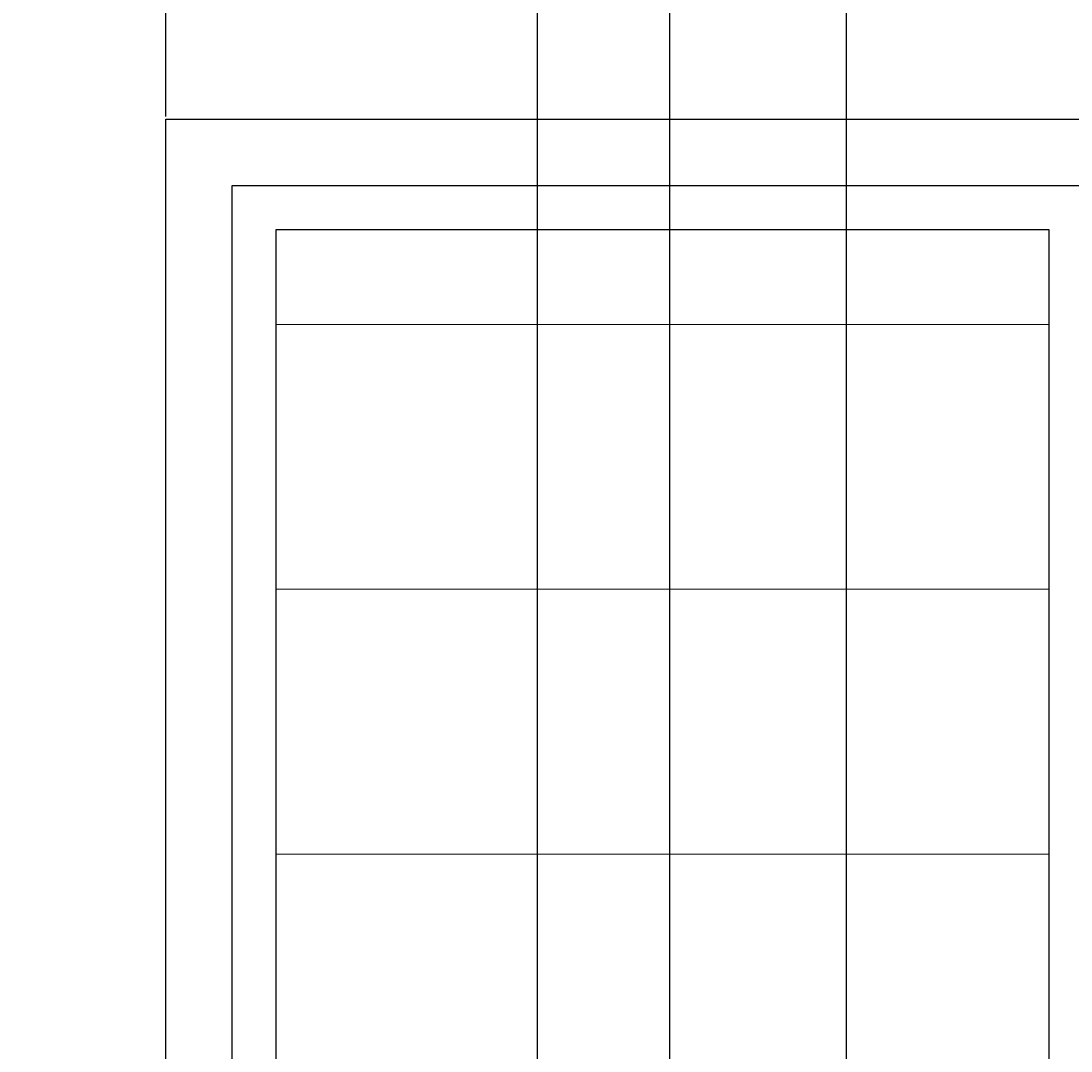
# Model space of a CAD drawing. Units: inches. Extents: x -6 to 289, y -8 to 323.
# Tile 59 of 107: x 124 to 147, y 206 to 229. Entities that reach past the tile are written whole.
import ezdxf

# ---------------------------------------------------------------- set-up
doc = ezdxf.new("R2010")
doc.units = ezdxf.units.IN
doc.header["$MEASUREMENT"] = 0
for name, color, linetype, lineweight in [('A-ANNO-DIMS', 2, 'Continuous', 18), ('A-ELEV-PATT', 8, 'Continuous', 13), ('A-GLAZ', 4, 'Continuous', 25)]:
    doc.layers.add(name, color=color, linetype=linetype, lineweight=lineweight)
doc.styles.get("Standard").update_dxf_attribs({"font": 'arial.ttf'})
doc.dimstyles.get("Standard").update_dxf_attribs({"dimtxt": 0.18, "dimasz": 0.18, "dimexe": 0.18, "dimexo": 0.0625, "dimgap": 0.09, "dimtad": 0, "dimtih": 1, "dimtoh": 1, "dimdec": 4, "dimzin": 0, "dimdsep": 46, "dimtxsty": 'Standard', "dimcen": 0.09, "dimadec": 0, "dimazin": 0, "dimtfac": 1, "dimtdec": 4, "dimtofl": 0, "dimtmove": 0, "dimatfit": 3, "dimfxl": 1, "dimtolj": 1, "dimtzin": 0, "dimarcsym": 0})

# ---------------------------------------------------------------- blocks, each defined once
blk = doc.blocks.new('*U4')
for p, q in [((1.5, 1.5), (1.5, 46.5)), ((1.5, 46.5), (21, 46.5))]:
    blk.add_line(p, q)
blk.add_lwpolyline([(0, 0), (0, 48), (42, 48), (42, 0)], close=True)
blk.add_lwpolyline([(20, 45.5), (20, 2.5), (2.5, 2.5), (2.5, 45.5), (20, 45.5)])
blk = doc.blocks.new('*D10')
at = {"layer": 'A-ANNO-DIMS', "color": 0, "lineweight": -2, "transparency": 16777216}
for p, q in [((115.164, 307.351), (115.164, 322.969)), ((115.344, 322.789), (120.639, 322.789)), ((126.703, 322.789), (121.408, 322.789)), ((126.883, 226.717), (126.883, 322.969))]:
    blk.add_line(p, q, dxfattribs=at)
at = {"layer": 'A-ANNO-DIMS', "color": 0, "transparency": 16777216}
for points in [[(115.344, 322.819), (115.344, 322.759), (115.164, 322.789)], [(126.703, 322.819), (126.703, 322.759), (126.883, 322.789)]]:
    blk.add_solid(points, dxfattribs=at)
at = {"layer": 'Defpoints', "color": 0, "transparency": 16777216}
for p in [(126.883, 322.789), (115.164, 307.289), (126.883, 226.654)]:
    blk.add_point(p, dxfattribs=at)
at = {"layer": 'A-ANNO-DIMS', "color": 0, "transparency": 16777216, "insert": (121.024, 322.789), "char_height": 0.18, "attachment_point": 5}
blk.add_mtext('\\A1;11.72', dxfattribs=at)
blk = doc.blocks.new('*D11')
at = {"layer": 'A-ANNO-DIMS', "color": 0, "lineweight": -2, "transparency": 16777216}
for p, q in [((126.883, 226.717), (126.883, 322.969)), ((127.063, 322.789), (147.662, 322.789)), ((168.703, 322.789), (148.105, 322.789)), ((168.883, 226.717), (168.883, 322.969))]:
    blk.add_line(p, q, dxfattribs=at)
at = {"layer": 'A-ANNO-DIMS', "color": 0, "transparency": 16777216}
for points in [[(127.063, 322.819), (127.063, 322.759), (126.883, 322.789)], [(168.703, 322.819), (168.703, 322.759), (168.883, 322.789)]]:
    blk.add_solid(points, dxfattribs=at)
at = {"layer": 'Defpoints', "color": 0, "transparency": 16777216}
for p in [(168.883, 322.789), (126.883, 226.654), (168.883, 226.654)]:
    blk.add_point(p, dxfattribs=at)
at = {"layer": 'A-ANNO-DIMS', "color": 0, "transparency": 16777216, "insert": (147.883, 322.789), "char_height": 0.18, "attachment_point": 5}
blk.add_mtext('\\A1;42', dxfattribs=at)
blk = doc.blocks.new('*D25')
at = {"layer": 'A-ANNO-DIMS', "color": 0, "lineweight": -2, "transparency": 16777216}
for p, q in [((126.946, 226.654), (288.653, 226.654)), ((288.473, 226.474), (288.473, 202.836)), ((288.473, 178.834), (288.473, 202.472)), ((126.946, 178.654), (288.653, 178.654))]:
    blk.add_line(p, q, dxfattribs=at)
at = {"layer": 'A-ANNO-DIMS', "color": 0, "transparency": 16777216}
for points in [[(288.443, 226.474), (288.503, 226.474), (288.473, 226.654)], [(288.443, 178.834), (288.503, 178.834), (288.473, 178.654)]]:
    blk.add_solid(points, dxfattribs=at)
at = {"layer": 'Defpoints', "color": 0, "transparency": 16777216}
for p in [(126.883, 226.654), (288.473, 226.654), (126.883, 178.654)]:
    blk.add_point(p, dxfattribs=at)
at = {"layer": 'A-ANNO-DIMS', "color": 0, "transparency": 16777216, "insert": (288.473, 202.654), "char_height": 0.18, "attachment_point": 5}
blk.add_mtext('\\A1;48', dxfattribs=at)
blk = doc.blocks.new('*D26')
at = {"layer": 'A-ANNO-DIMS', "color": 0, "lineweight": -2, "transparency": 16777216}
for p, q in [((247.226, 247.289), (288.653, 247.289)), ((288.473, 247.109), (288.473, 237.153)), ((288.473, 226.834), (288.473, 236.789)), ((126.946, 226.654), (288.653, 226.654))]:
    blk.add_line(p, q, dxfattribs=at)
at = {"layer": 'A-ANNO-DIMS', "color": 0, "transparency": 16777216}
for points in [[(288.443, 247.109), (288.503, 247.109), (288.473, 247.289)], [(288.443, 226.834), (288.503, 226.834), (288.473, 226.654)]]:
    blk.add_solid(points, dxfattribs=at)
at = {"layer": 'Defpoints', "color": 0, "transparency": 16777216}
for p in [(247.164, 247.289), (288.473, 247.289), (126.883, 226.654)]:
    blk.add_point(p, dxfattribs=at)
at = {"layer": 'A-ANNO-DIMS', "color": 0, "transparency": 16777216, "insert": (288.473, 236.971), "char_height": 0.18, "attachment_point": 5}
blk.add_mtext('\\A1;20.635', dxfattribs=at)
blk = doc.blocks.new('*D73')
at = {"layer": 'A-ANNO-DIMS', "color": 0, "lineweight": -2, "transparency": 16777216}
for p, q in [((121.008, 51.148), (121.008, 322.969)), ((121.188, 322.789), (127.697, 322.789)), ((135.116, 322.789), (128.607, 322.789)), ((135.296, 51.148), (135.296, 322.969))]:
    blk.add_line(p, q, dxfattribs=at)
at = {"layer": 'A-ANNO-DIMS', "color": 0, "transparency": 16777216}
for points in [[(121.188, 322.819), (121.188, 322.759), (121.008, 322.789)], [(135.116, 322.819), (135.116, 322.759), (135.296, 322.789)]]:
    blk.add_solid(points, dxfattribs=at)
at = {"layer": 'Defpoints', "color": 0, "transparency": 16777216}
for p in [(135.296, 322.789), (121.008, 51.085), (135.296, 51.085)]:
    blk.add_point(p, dxfattribs=at)
at = {"layer": 'A-ANNO-DIMS', "color": 0, "transparency": 16777216, "insert": (128.152, 322.789), "char_height": 0.18, "attachment_point": 5}
blk.add_mtext('\\A1;14.288', dxfattribs=at)
blk = doc.blocks.new('*D74')
at = {"layer": 'A-ANNO-DIMS', "color": 0, "lineweight": -2, "transparency": 16777216}
for p, q in [((135.296, 51.148), (135.296, 322.969)), ((135.476, 322.789), (136.647, 322.789)), ((138.116, 322.789), (136.945, 322.789)), ((138.296, 51.148), (138.296, 322.969))]:
    blk.add_line(p, q, dxfattribs=at)
at = {"layer": 'A-ANNO-DIMS', "color": 0, "transparency": 16777216}
for points in [[(135.476, 322.819), (135.476, 322.759), (135.296, 322.789)], [(138.116, 322.819), (138.116, 322.759), (138.296, 322.789)]]:
    blk.add_solid(points, dxfattribs=at)
at = {"layer": 'Defpoints', "color": 0, "transparency": 16777216}
for p in [(138.296, 322.789), (135.296, 51.085), (138.296, 51.085)]:
    blk.add_point(p, dxfattribs=at)
at = {"layer": 'A-ANNO-DIMS', "color": 0, "transparency": 16777216, "insert": (136.796, 322.789), "char_height": 0.18, "attachment_point": 5}
blk.add_mtext('\\A1;3', dxfattribs=at)
blk = doc.blocks.new('*D75')
at = {"layer": 'A-ANNO-DIMS', "color": 0, "lineweight": -2, "transparency": 16777216}
for p, q in [((138.296, 51.148), (138.296, 322.969)), ((138.476, 322.789), (140.144, 322.789)), ((142.116, 322.789), (140.448, 322.789)), ((142.296, 51.148), (142.296, 322.969))]:
    blk.add_line(p, q, dxfattribs=at)
at = {"layer": 'A-ANNO-DIMS', "color": 0, "transparency": 16777216}
for points in [[(138.476, 322.819), (138.476, 322.759), (138.296, 322.789)], [(142.116, 322.819), (142.116, 322.759), (142.296, 322.789)]]:
    blk.add_solid(points, dxfattribs=at)
at = {"layer": 'Defpoints', "color": 0, "transparency": 16777216}
for p in [(142.296, 322.789), (138.296, 51.085), (142.296, 51.085)]:
    blk.add_point(p, dxfattribs=at)
at = {"layer": 'A-ANNO-DIMS', "color": 0, "transparency": 16777216, "insert": (140.296, 322.789), "char_height": 0.18, "attachment_point": 5}
blk.add_mtext('\\A1;4', dxfattribs=at)
blk = doc.blocks.new('*D76')
at = {"layer": 'A-ANNO-DIMS', "color": 0, "lineweight": -2, "transparency": 16777216}
for p, q in [((142.296, 51.148), (142.296, 322.969)), ((142.476, 322.789), (153.076, 322.789)), ((164.116, 322.789), (153.516, 322.789)), ((164.296, 51.148), (164.296, 322.969))]:
    blk.add_line(p, q, dxfattribs=at)
at = {"layer": 'A-ANNO-DIMS', "color": 0, "transparency": 16777216}
for points in [[(142.476, 322.819), (142.476, 322.759), (142.296, 322.789)], [(164.116, 322.819), (164.116, 322.759), (164.296, 322.789)]]:
    blk.add_solid(points, dxfattribs=at)
at = {"layer": 'Defpoints', "color": 0, "transparency": 16777216}
for p in [(164.296, 322.789), (142.296, 51.085), (164.296, 51.085)]:
    blk.add_point(p, dxfattribs=at)
at = {"layer": 'A-ANNO-DIMS', "color": 0, "transparency": 16777216, "insert": (153.296, 322.789), "char_height": 0.18, "attachment_point": 5}
blk.add_mtext('\\A1;22', dxfattribs=at)
blk = doc.blocks.new('*D94')
at = {"layer": 'A-ANNO-DIMS', "color": 0, "lineweight": -2, "transparency": 16777216}
for p, q in [((118.164, 159.411), (118.164, 322.969)), ((118.344, 322.789), (139.46, 322.789)), ((161.372, 322.789), (140.256, 322.789)), ((161.552, 159.411), (161.552, 322.969))]:
    blk.add_line(p, q, dxfattribs=at)
at = {"layer": 'A-ANNO-DIMS', "color": 0, "transparency": 16777216}
for points in [[(118.344, 322.819), (118.344, 322.759), (118.164, 322.789)], [(161.372, 322.819), (161.372, 322.759), (161.552, 322.789)]]:
    blk.add_solid(points, dxfattribs=at)
at = {"layer": 'Defpoints', "color": 0, "transparency": 16777216}
for p in [(161.552, 322.789), (118.164, 159.348), (161.552, 159.348)]:
    blk.add_point(p, dxfattribs=at)
at = {"layer": 'A-ANNO-DIMS', "color": 0, "transparency": 16777216, "insert": (139.858, 322.789), "char_height": 0.18, "attachment_point": 5}
blk.add_mtext('\\A1;43.39', dxfattribs=at)

msp = doc.modelspace()

# ---------------------------------------------------------------- hatches: boundary and pattern name
at = {"layer": 'A-ELEV-PATT'}
h = msp.add_hatch(dxfattribs=at)
h.set_pattern_fill('_USER', color=256, scale=6, pattern_type=0)
h.set_pattern_definition([(0, (0, 0), (0, 6), [])])
h.paths.add_polyline_path([(184.1244, 48.0851), (124.008, 48.0851), (124.008, 10.2888), (184.1244, 10.2888)])
h.paths.add_polyline_path([(244.2408, 48.0851), (186.3604, 48.0851), (186.3604, 10.2888), (244.2408, 10.2888)])
h.paths.add_polyline_path([(208.2918, 114.2795), (190.7918, 114.2795), (190.7918, 71.2795), (208.2918, 71.2795)])
h.paths.add_polyline_path([(227.7918, 114.2795), (209.2918, 114.2795), (209.2918, 71.2795), (227.7918, 71.2795)])
h.paths.add_polyline_path([(211.2918, 224.3887), (190.7918, 224.3887), (190.7918, 162.3484), (211.2918, 162.3484)])
h.paths.add_polyline_path([(233.7918, 224.3887), (212.2918, 224.3887), (212.2918, 162.3484), (233.7918, 162.3484)])
h.paths.add_polyline_path([(166.3835, 224.154), (147.8835, 224.154), (147.8835, 181.154), (166.3835, 181.154)])
h.paths.add_polyline_path([(146.8835, 224.154), (129.3835, 224.154), (129.3835, 181.154), (146.8835, 181.154)])

# ---------------------------------------------------------------- block references
at = {"layer": 'A-GLAZ'}
msp.add_blockref('*U4', (126.8835, 178.654), dxfattribs=at)

# ---------------------------------------------------------------- dimensions: what is measured, and where the dimension line sits
at = {"layer": 'A-ANNO-DIMS'}
for base, p1, p2, override, picture, middle in [((126.8835, 322.7888), (115.1638, 307.2888), (126.8835, 226.654), {"dimdec": 2, "dimlfac": 1, "dimrnd": 0, "dimzin": 0, "dimdsep": 46, "dimlunit": 2}, '*D10', (121.0236, 322.7888)), ((161.5522, 322.7888), (118.1638, 159.3484), (161.5522, 159.3484), {"dimdec": 2, "dimlfac": 1, "dimrnd": 0, "dimzin": 0, "dimdsep": 46, "dimlunit": 2}, '*D94', (139.858, 322.7888)), ((135.296, 322.7888), (121.008, 51.0851), (135.296, 51.0851), {"dimdec": 3, "dimlfac": 1, "dimrnd": 0, "dimzin": 0, "dimdsep": 46, "dimlunit": 2}, '*D73', (128.152, 322.7888)), ((168.8835, 322.7888), (126.8835, 226.654), (168.8835, 226.654), {"dimdec": 0, "dimlfac": 1, "dimrnd": 0, "dimzin": 0, "dimdsep": 46, "dimlunit": 2}, '*D11', (147.8835, 322.7888)), ((138.296, 322.7888), (135.296, 51.0851), (138.296, 51.0851), {"dimdec": 0, "dimlfac": 1, "dimrnd": 0, "dimzin": 0, "dimdsep": 46, "dimlunit": 2}, '*D74', (136.796, 322.7888)), ((142.296, 322.7888), (138.296, 51.0851), (142.296, 51.0851), {"dimdec": 0, "dimlfac": 1, "dimrnd": 0, "dimzin": 0, "dimdsep": 46, "dimlunit": 2}, '*D75', (140.296, 322.7888)), ((164.296, 322.7888), (142.296, 51.0851), (164.296, 51.0851), {"dimdec": 0, "dimlfac": 1, "dimrnd": 0, "dimzin": 0, "dimdsep": 46, "dimlunit": 2}, '*D76', (153.296, 322.7888))]:
    dim = msp.add_linear_dim(base=base, p1=p1, p2=p2, dimstyle='Standard', override=override, dxfattribs=at)
    dim.commit()
    dim.dimension.update_dxf_attribs({"geometry": picture, "text_midpoint": middle})
for base, p1, p2, override, picture, middle in [((288.4733, 247.2888), (126.8835, 226.654), (247.1638, 247.2888), {"dimdec": 3, "dimlfac": 1, "dimrnd": 0, "dimzin": 0, "dimdsep": 46, "dimlunit": 2}, '*D26', (288.4733, 236.9714)), ((288.4733, 226.654), (126.8835, 178.654), (126.8835, 226.654), {"dimdec": 0, "dimlfac": 1, "dimrnd": 0, "dimzin": 0, "dimdsep": 46, "dimlunit": 2}, '*D25', (288.4733, 202.654))]:
    dim = msp.add_linear_dim(base=base, p1=p1, p2=p2, angle=90, dimstyle='Standard', override=override, dxfattribs=at)
    dim.commit()
    dim.dimension.update_dxf_attribs({"geometry": picture, "text_midpoint": middle})

doc.saveas('drawing.dxf')
